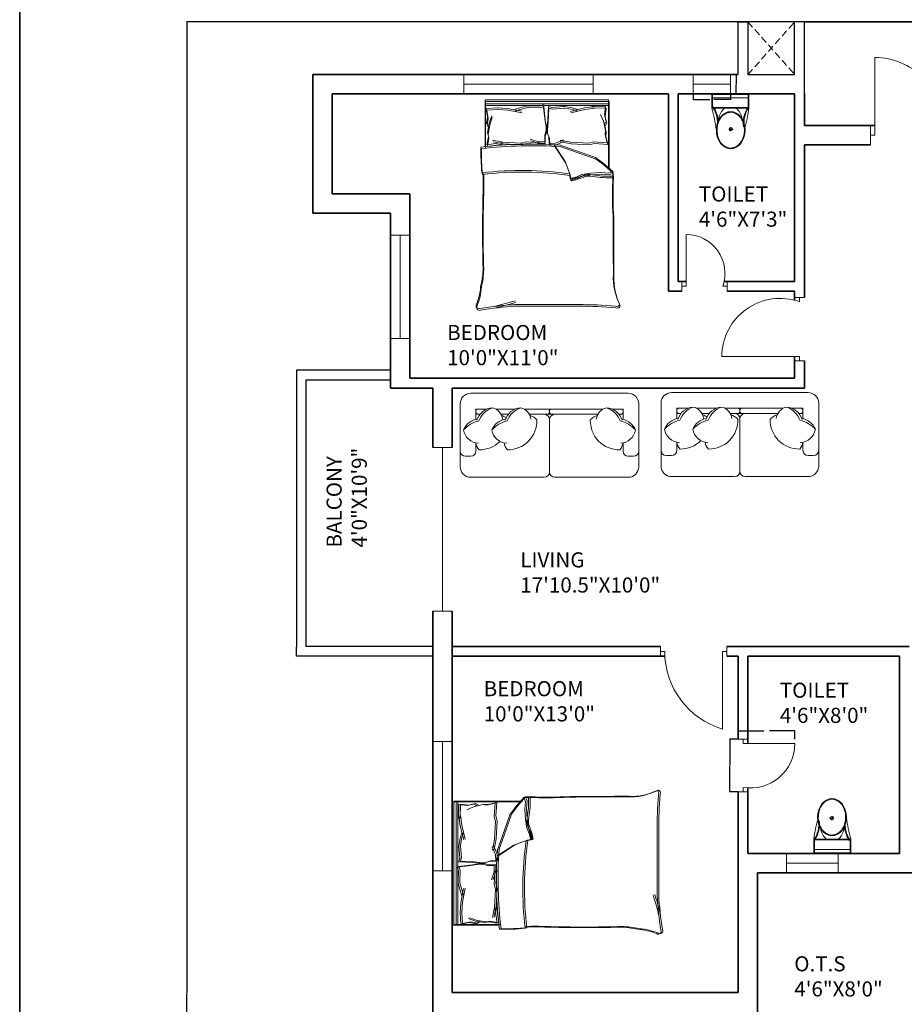
# Model space of a CAD drawing. Units: inches. Extents: x 2296 to 3812, y -1531 to 2564.
# Tile 3 of 10: x 2296 to 2706, y 1719 to 2176. Entities that reach past the tile are written whole.
import ezdxf

# ---------------------------------------------------------------- set-up
doc = ezdxf.new("R2010")
doc.units = ezdxf.units.IN
doc.linetypes.add('HIDDEN2', pattern=[4.7625, 3.175, -1.5875])
for name, color, linetype, lineweight in [('A-ANNO-DIMS', 2, 'Continuous', 18), ('A-ANNO-TTLB', 7, 'Continuous', 35), ('A-AREA-IDEN', 7, 'Continuous', 18), ('A-DOOR', 3, 'Continuous', 18), ('A-FLOR-FIXT', 9, 'Continuous', 18), ('A-FLOR-HRAL', 7, 'Continuous', 25), ('A-FURN', 8, 'Continuous', 18), ('A-GLAZ', 4, 'Continuous', 18), ('A-WALL', 7, 'Continuous', 35), ('A-WALL-HIDN', 8, 'HIDDEN2', 18)]:
    doc.layers.add(name, color=color, linetype=linetype, lineweight=lineweight)
doc.styles.get("Standard").update_dxf_attribs({"font": 'arial.ttf'})
doc.dimstyles.get("Standard").update_dxf_attribs({"dimtxt": 0.18, "dimasz": 0.18, "dimexe": 0.18, "dimexo": 0.0625, "dimgap": 0.09, "dimtad": 0, "dimtih": 1, "dimtoh": 1, "dimdec": 4, "dimzin": 0, "dimdsep": 46, "dimtxsty": 'Standard', "dimcen": 0.09, "dimadec": 0, "dimazin": 0, "dimtfac": 1, "dimtdec": 4, "dimtofl": 0, "dimtmove": 0, "dimatfit": 3, "dimfxl": 1, "dimtolj": 1, "dimtzin": 0, "dimarcsym": 0})

# ---------------------------------------------------------------- blocks, each defined once
blk = doc.blocks.new('A$C31115884')
for p, q in [((283, 498), (223, 498)), ((258, 466), (258, 523)), ((0, 200), (0, 0)), ((520, 200), (0, 200)), ((10, 190), (10, 10)), ((510, 190), (10, 190)), ((510, 10), (510, 190)), ((520, 0), (520, 200)), ((510, 54), (0, 54)), ((10, 10), (510, 10)), ((0, 0), (520, 0))]:
    blk.add_line(p, q)
blk.add_circle((256, 496), 23.6)
for centre, radius, start, end in [((2778, -205), 2807, 165.4549, 171.7133), ((-295, 403), 365, 324.2091, 9.3499), ((-295, 403), 375, 324.2091, 9.3499), ((139, 406), 293, 315.8436, 2.6563), ((806, 403), 365, 170.6501, 215.7909), ((3237, 905), 2807, 188.2867, 194.5451), ((384, 406), 293, 190.2774, 224.1564), ((806, 403), 375, 179.2036, 215.7909)]:
    blk.add_arc(centre, radius, start, end)
blk.add_ellipse((256, 510), major_axis=(0, -261), ratio=0.772727)
blk.add_open_spline([(256, 259), (263, 259), (270, 260), (288, 262), (299, 265), (320, 273), (330, 278), (350, 291), (360, 299), (378, 316), (386, 326), (402, 347), (409, 358), (421, 383), (427, 395), (436, 422), (440, 436), (445, 465), (447, 480), (448, 509), (448, 524), (445, 553), (443, 568), (436, 596), (432, 610), (422, 636), (416, 649), (402, 672), (395, 683), (379, 703), (370, 712), (351, 728), (341, 735), (321, 746), (310, 751), (289, 757), (278, 759), (256, 761), (245, 761), (223, 757), (212, 754), (191, 746), (181, 741), (161, 728), (151, 720), (133, 703), (125, 693), (110, 672), (103, 660), (90, 636), (85, 623), (76, 596), (72, 582), (67, 553), (66, 538), (64, 509), (65, 494), (68, 465), (70, 450), (77, 422), (81, 408), (91, 382), (97, 370), (111, 346), (118, 335), (135, 316), (144, 307), (162, 291), (172, 284), (193, 273), (203, 269), (225, 262), (236, 260), (250, 259), (253, 259), (256, 259)], degree=3, knots=[0, 0, 0, 0, 0.110105, 0.110105, 0.285049, 0.285049, 0.459994, 0.459994, 0.634938, 0.634938, 0.809882, 0.809882, 0.984827, 0.984827, 1.159771, 1.159771, 1.334715, 1.334715, 1.50966, 1.50966, 1.684604, 1.684604, 1.859549, 1.859549, 2.034493, 2.034493, 2.209437, 2.209437, 2.384382, 2.384382, 2.559326, 2.559326, 2.73427, 2.73427, 2.909215, 2.909215, 3.084159, 3.084159, 3.259103, 3.259103, 3.434048, 3.434048, 3.608992, 3.608992, 3.783936, 3.783936, 3.958881, 3.958881, 4.133825, 4.133825, 4.30877, 4.30877, 4.483714, 4.483714, 4.658658, 4.658658, 4.833603, 4.833603, 5.008547, 5.008547, 5.183491, 5.183491, 5.358436, 5.358436, 5.53338, 5.53338, 5.708324, 5.708324, 5.883269, 5.883269, 6.058213, 6.058213, 6.233158, 6.233158, 6.283185, 6.283185, 6.283185, 6.283185])
blk = doc.blocks.new('DOOR-BEDROOM-ENTRY-NW')
for p, q in [((33.75, 29.46), (38.25, 29.46)), ((38.25, 29.46), (36, 29.46)), ((36, 29.46), (36, 27.46)), ((36, 2), (0, 2)), ((33.75, 0), (38.25, 0)), ((36, 0), (36, 2)), ((38.25, 0), (36, 0))]:
    blk.add_line(p, q)
blk.add_arc((27, 2), 27, 70.5334, 180)
blk = doc.blocks.new('DOOR-BATH-24-NW')
for p, q in [((2, 2.25), (2, 26.25)), ((0, 4.5), (0, 0)), ((0, 0), (0, 2.25)), ((0, 2.25), (2, 2.25)), ((21.01, 2.25), (19.01, 2.25)), ((21.01, 4.5), (21.01, 0)), ((21.01, 0), (21.01, 2.25))]:
    blk.add_line(p, q)
blk.add_arc((2, 8.22), 18.03, 340.6613, 90)
blk = doc.blocks.new('DOOR-BALCONY-PAIR-N')
for p, q in [((2, 4.5), (2, 40.5)), ((64.91, 4.5), (64.91, 40.5)), ((0, 9), (0, 0)), ((66.91, 9), (66.91, 0)), ((0, 0), (0, 4.5)), ((0, 4.5), (2, 4.5)), ((66.91, 4.5), (64.91, 4.5)), ((66.91, 0), (66.91, 4.5))]:
    blk.add_line(p, q)
for centre, radius, start, end in [((2, 9.22), 31.28, 359.5901, 90), ((64.41, 9.36), 31.14, 89.0831, 180.6679)]:
    blk.add_arc(centre, radius, start, end)
blk = doc.blocks.new('DOOR-BEDROOM-36-WN')
for p, q in [((0, 38.25), (0, 33.75)), ((30.77, 38.25), (30.77, 33.75)), ((0, 33.75), (0, 36)), ((0, 36), (2, 36)), ((30.77, 36), (28.77, 36)), ((28.77, 36), (28.77, 0)), ((30.77, 33.75), (30.77, 36))]:
    blk.add_line(p, q)
blk.add_arc((39.59, 36), 37.59, 180, 253.2783)
blk = doc.blocks.new('DOOR-BATH-24-WN')
for p, q in [((0, 24.31), (4.5, 24.31)), ((4.5, 24.31), (2.25, 24.31)), ((2.25, 24.31), (2.25, 22.31)), ((2.25, 22.31), (26.25, 22.31)), ((2.25, 0), (2.25, 2)), ((4.5, 0), (0, 0)), ((0, 0), (2.25, 0))]:
    blk.add_line(p, q)
blk.add_arc((5.66, 22.31), 20.59, 260.4824, 0)
blk = doc.blocks.new('WIN-60-BEDROOM-N')
for p, q in [((0, 9), (0, 0)), ((60, 4.5), (60, 9)), ((60, 9), (60, 0)), ((0, 0), (0, 4.5)), ((0, 4.5), (60, 4.5)), ((60, 4.5), (60, 4.5))]:
    blk.add_line(p, q)
blk = doc.blocks.new('WIN-24-SHAFT-N')
for p, q in [((0, 9), (0, 0)), ((24, 4.5), (24, 9)), ((24, 9), (24, 9)), ((24, 9), (24, 0)), ((0, 0), (0, 4.5)), ((0, 4.5), (24, 4.5))]:
    blk.add_line(p, q)
blk = doc.blocks.new('WIN-60-JAMB-B')
for p, q in [((0, 60), (9, 60)), ((9, 60), (4.5, 60)), ((4.5, 60), (4.5, 0)), ((4.5, 0), (0, 0)), ((0, 0), (9, 0))]:
    blk.add_line(p, q)
blk = doc.blocks.new('WIN-17-VENT')
for p, q in [((0, 9), (0, 0)), ((17.26, 4.5), (17.26, 9)), ((17.26, 7.76), (17.26, 0)), ((0, 0), (0, 4.5)), ((0, 4.5), (0, 4.5)), ((0, 4.5), (17.26, 4.5))]:
    blk.add_line(p, q)
blk = doc.blocks.new('WIN-48-BEDROOM-NW')
for p, q in [((0, 48), (9, 48)), ((9, 48), (4.5, 48)), ((4.5, 48), (4.5, 0)), ((4.5, 0), (0, 0)), ((0, 0), (9, 0))]:
    blk.add_line(p, q)
blk = doc.blocks.new('GLAZ-BALCONY-N')
for p, q in [((0, 75.98), (9, 75.98)), ((4.5, 75.98), (4.5, 0)), ((0, 0), (9, 0))]:
    blk.add_line(p, q)
blk = doc.blocks.new('BED-DOUBLE')
for p, q in [((48.49, 95), (18.98, 95)), ((3.07, 35.36), (3.17, 33.26, 4.64)), ((5.01, 34.01), (3.17, 33.26)), ((3.17, 33.26), (7.61, 29.37)), ((8.72, 33.63), (5.01, 34.01)), ((13.37, 34.01), (8.72, 33.63)), ((17.45, 34.56), (13.37, 34.01)), ((19.86, 35.68), (17.45, 34.56)), ((22.83, 36.42), (19.86, 35.68)), ((23.21, 34.01), (22.83, 36.42)), ((25.25, 28.62), (23.21, 34.01)), ((5.09, 0), (5.09, 31.9)), ((7.61, 29.37), (11.14, 26.77)), ((30.27, 20.84), (25.25, 28.62)), ((11.14, 26.77), (17.82, 24.36)), ((17.82, 24.36), (27.82, 20.84)), ((11.92, 19.38), (5.77, 19.87)), ((5.77, 19.87), (6.7, 16.11)), ((14.27, 20.05), (11.92, 19.38)), ((22.67, 19.54), (14.27, 20.05)), ((27.51, 18.74), (22.67, 19.54)), ((29.68, 20.07), (26, 18.53)), ((32.62, 20.25), (29.68, 20.07)), ((32.82, 17.04), (32.62, 20.25)), ((34.71, 16.28), (34.71, 19.5)), ((34.71, 19.5), (37.65, 19.5)), ((43.31, 19.38), (37.16, 19.87)), ((37.65, 19.5), (41.42, 18.19)), ((45.66, 20.05), (43.31, 19.38)), ((54.06, 19.54), (45.66, 20.05)), ((54.06, 19.54), (55.42, 19.92)), ((58.9, 18.74), (54.06, 19.54)), ((55.42, 19.92), (61.53, 20.79)), ((61.53, 20.79), (60.84, 16.98)), ((62.38, 21.71), (62.38, 0)), ((6.7, 16.11), (6.47, 14.18)), ((6.47, 14.18), (7.43, 9.9)), ((33.66, 14.84), (32.82, 17.04)), ((33.75, 13.28), (33.66, 14.84)), ((34.01, 14.03), (34.71, 16.28)), ((34.01, 12.47), (34.01, 14.03)), ((61.19, 15.07), (60.49, 10.74)), ((60.84, 16.98), (61.19, 15.07)), ((6.21, 10), (6.83, 11.25)), ((6.93, 6.92), (6.21, 10)), ((7.43, 9.9), (8.85, 6.69)), ((33.01, 2.99), (33.3, 9.43)), ((33.3, 9.43), (33.75, 13.28)), ((34.71, 8.66), (34.01, 12.47)), ((60.49, 10.74), (59.28, 7.44)), ((61.71, 10.91), (61.01, 12.12)), ((61.19, 7.79), (61.71, 10.91)), ((6.47, 3.07), (6.93, 6.92)), ((16.3, 3.68), (22.8, 5.3)), ((35.4, 2.24), (34.71, 8.66)), ((52.03, 3.98), (45.45, 5.19)), ((61.88, 3.98), (61.19, 7.79)), ((62.38, 1.84), (5.09, 1.84)), ((62.38, 0), (5.09, 0)), ((6.47, 3.07), (12.95, 2.95)), ((11.75, 3.05), (16.3, 3.68)), ((12.95, 2.95), (11.75, 3.05)), ((19.55, 4.4), (22.03, 3.69)), ((22.03, 3.69), (25.54, 3.04)), ((25.54, 3.04), (25.93, 3.07)), ((25.93, 3.07), (31.24, 3.57)), ((31.24, 3.57), (33.01, 2.99)), ((37.13, 2.94), (35.4, 2.24)), ((42.46, 2.76), (37.13, 2.94)), ((42.85, 2.76), (42.46, 2.76)), ((46.31, 3.63), (42.85, 2.76)), ((48.74, 4.5), (46.31, 3.63)), ((56.62, 3.63), (52.03, 3.98)), ((56.74, 3.61), (56.62, 3.63)), ((61.87, 4), (56.74, 3.61))]:
    blk.add_line(p, q)
for centre, radius, start, end in [((40.86, 240.78), 145.97, 272.9958, 279.4091), ((65.24, 95.57), 1.31, 326.1736, 113.4781), ((1.32, 94.55), 1.32, 62.6588, 176.02), ((-24.75, 82.32), 27.65, 357.4714, 26.4681), ((17.21, 254.49), 159.5, 264.4998, 270.6351), ((87.19, -28.43), 127.63, 103.3832, 107.7053), ((92.52, 84.25), 28.25, 157.9751, 176.652), ((98.8, 77.34), 35.53, 166.0648, 178.9113), ((5471.89, 81.31), 5469.02, 180.00217, 180.28689), ((-514.68, 60.68), 578.22, 358.22771, 1.71854), ((-151.96, 43.54), 155.25, 356.9791, 3.8365), ((267.13, 37.37), 203.94, 178.4762, 181.0082), ((29.2, 1.78), 35.55, 100.6617, 109.8806), ((22.63, 36.49), 0.221, 340.2464, 91.1377), ((5.01, -7.98), 43.38, 79.8763, 92.5657), ((14.11, 42.04), 7.46, 258.6608, 293.7384), ((45.26, 187.4), 154.68, 261.7845, 276.9006), ((-35.55, 24.09), 99.87, 358.7218, 5.604), ((40.94, 218.26), 197.77, 266.0865, 276.7821)]:
    blk.add_arc(centre, radius, start, end)
blk = doc.blocks.new('*D71')
at = {"layer": 'A-ANNO-DIMS', "color": 0, "lineweight": -2, "transparency": 16777216}
for p, q in [((2629.4, 1842.2), (2629.4, 1846.25)), ((2629.58, 1846.07), (2641.22, 1846.07)), ((2655.47, 1846.07), (2643.83, 1846.07)), ((2655.65, 1842.2), (2655.65, 1846.25))]:
    blk.add_line(p, q, dxfattribs=at)
at = {"layer": 'A-ANNO-DIMS', "color": 0, "transparency": 16777216}
for points in [[(2629.58, 1846.1), (2629.58, 1846.04), (2629.4, 1846.07)], [(2655.47, 1846.1), (2655.47, 1846.04), (2655.65, 1846.07)]]:
    blk.add_solid(points, dxfattribs=at)
at = {"layer": 'Defpoints', "color": 0, "transparency": 16777216}
for p in [(2655.65, 1846.07), (2629.4, 1842.13), (2655.65, 1842.13)]:
    blk.add_point(p, dxfattribs=at)
at = {"layer": 'A-ANNO-DIMS', "color": 0, "transparency": 16777216, "insert": (2642.53, 1846.07), "char_height": 0.18, "attachment_point": 5}
blk.add_mtext('\\A1;BATH DOOR 26 TYP.', dxfattribs=at)
blk = doc.blocks.new('*D72')
at = {"layer": 'A-ANNO-DIMS', "color": 0, "lineweight": -2, "transparency": 16777216}
for p, q in [((2629.34, 1842.13), (2625.28, 1842.13)), ((2625.46, 1841.95), (2625.46, 1830.16)), ((2625.46, 1818), (2625.46, 1829.8)), ((2629.34, 1817.82), (2625.28, 1817.82))]:
    blk.add_line(p, q, dxfattribs=at)
at = {"layer": 'A-ANNO-DIMS', "color": 0, "transparency": 16777216}
for points in [[(2625.43, 1841.95), (2625.49, 1841.95), (2625.46, 1842.13)], [(2625.43, 1818), (2625.49, 1818), (2625.46, 1817.82)]]:
    blk.add_solid(points, dxfattribs=at)
at = {"layer": 'Defpoints', "color": 0, "transparency": 16777216}
for p in [(2625.46, 1842.13), (2629.4, 1842.13), (2629.4, 1817.82)]:
    blk.add_point(p, dxfattribs=at)
at = {"layer": 'A-ANNO-DIMS', "color": 0, "transparency": 16777216, "insert": (2625.46, 1829.98), "char_height": 0.18, "attachment_point": 5}
blk.add_mtext('\\A1;24 TYP.', dxfattribs=at)
blk = doc.blocks.new('*D119')
at = {"layer": 'A-ANNO-DIMS', "color": 0, "lineweight": -2, "transparency": 16777216}
for p, q in [((2608.53, 2141.6), (2608.53, 2138.89)), ((2608.71, 2139.07), (2616.25, 2139.07)), ((2625.61, 2139.07), (2618.06, 2139.07)), ((2625.79, 2141.6), (2625.79, 2138.89))]:
    blk.add_line(p, q, dxfattribs=at)
at = {"layer": 'A-ANNO-DIMS', "color": 0, "transparency": 16777216}
for points in [[(2608.71, 2139.1), (2608.71, 2139.04), (2608.53, 2139.07)], [(2625.61, 2139.1), (2625.61, 2139.04), (2625.79, 2139.07)]]:
    blk.add_solid(points, dxfattribs=at)
at = {"layer": 'Defpoints', "color": 0, "transparency": 16777216}
for p in [(2608.53, 2141.66), (2625.79, 2141.66), (2625.79, 2139.07)]:
    blk.add_point(p, dxfattribs=at)
at = {"layer": 'A-ANNO-DIMS', "color": 0, "transparency": 16777216, "insert": (2617.16, 2139.07), "char_height": 0.18, "attachment_point": 5}
blk.add_mtext('\\A1;VENT 17 TYP.', dxfattribs=at)
blk = doc.blocks.new('*D120')
at = {"layer": 'A-ANNO-DIMS', "color": 0, "lineweight": -2, "transparency": 16777216}
for p, q in [((2625.85, 2150.66), (2628.56, 2150.66)), ((2628.38, 2150.48), (2628.38, 2146.34)), ((2628.38, 2141.84), (2628.38, 2145.98)), ((2625.85, 2141.66), (2628.56, 2141.66))]:
    blk.add_line(p, q, dxfattribs=at)
at = {"layer": 'A-ANNO-DIMS', "color": 0, "transparency": 16777216}
for points in [[(2628.35, 2150.48), (2628.41, 2150.48), (2628.38, 2150.66)], [(2628.35, 2141.84), (2628.41, 2141.84), (2628.38, 2141.66)]]:
    blk.add_solid(points, dxfattribs=at)
at = {"layer": 'Defpoints', "color": 0, "transparency": 16777216}
for p in [(2625.79, 2150.66), (2628.38, 2150.66), (2625.79, 2141.66)]:
    blk.add_point(p, dxfattribs=at)
at = {"layer": 'A-ANNO-DIMS', "color": 0, "transparency": 16777216, "insert": (2628.38, 2146.16), "char_height": 0.18, "attachment_point": 5}
blk.add_mtext('\\A1;9 TYP.', dxfattribs=at)
blk = doc.blocks.new('*D128')
at = {"layer": 'A-ANNO-DIMS', "color": 0, "lineweight": -2, "transparency": 16777216}
for p, q in [((2660.01, 2175.03), (2373.54, 2175.03)), ((2373.72, 2174.85), (2373.72, 1724.41)), ((2373.72, 1273.61), (2373.72, 1724.05)), ((2666.19, 1273.43), (2373.54, 1273.43))]:
    blk.add_line(p, q, dxfattribs=at)
at = {"layer": 'A-ANNO-DIMS', "color": 0, "transparency": 16777216}
for points in [[(2373.69, 2174.85), (2373.75, 2174.85), (2373.72, 2175.03)], [(2373.69, 1273.61), (2373.75, 1273.61), (2373.72, 1273.43)]]:
    blk.add_solid(points, dxfattribs=at)
at = {"layer": 'Defpoints', "color": 0, "transparency": 16777216}
for p in [(2373.72, 2175.03), (2660.07, 2175.03), (2666.25, 1273.43)]:
    blk.add_point(p, dxfattribs=at)
at = {"layer": 'A-ANNO-DIMS', "color": 0, "transparency": 16777216, "insert": (2373.72, 1724.23), "char_height": 0.18, "attachment_point": 5}
blk.add_mtext('\\A1;901.6', dxfattribs=at)

msp = doc.modelspace()

# ---------------------------------------------------------------- linework, layer by layer
at = {"layer": 'A-ANNO-TTLB'}
msp.add_lwpolyline([(2296.1257, 2564.2989), (3812.4193, 2564.2989), (3812.4193, 1124.0028), (2296.1257, 1124.0028)], close=True, dxfattribs=at)
at = {"layer": 'A-FLOR-HRAL'}
for p, q in [((2629.4179, 2150.6578), (2629.4179, 2175.0276)), ((2629.4179, 2175.0276), (2633.9179, 2175.0276)), ((2633.9179, 2175.0276), (2633.9179, 2150.6578)), ((2655.5693, 2150.6578), (2655.5693, 2175.0276)), ((2789.0693, 2175.0276), (2655.5693, 2175.0276)), ((2660.0693, 2141.6578), (2660.0693, 2175.0276)), ((2660.0693, 2127.0276), (2660.0693, 2175.0276)), ((2660.0693, 2175.0276), (2789.0693, 2175.0276)), ((2633.9179, 2150.6578), (2655.5693, 2150.6578)), ((2633.9179, 2150.6578), (2655.5693, 2150.6578)), ((2468.0693, 2013.471), (2424.5693, 2013.471)), ((2424.5693, 2013.471), (2424.5693, 1884.8249)), ((2429.0693, 1889.3249), (2429.0693, 2008.971)), ((2429.0693, 2008.971), (2468.0693, 2008.971)), ((2429.0693, 1885.1578), (2429.0693, 1889.3249)), ((2424.5693, 1880.6578), (2424.5693, 1884.8249)), ((2487.7523, 1885.1578), (2429.0693, 1885.1578)), ((2487.7523, 1880.6578), (2424.5693, 1880.6578))]:
    msp.add_line(p, q, dxfattribs=at)
at = {"layer": 'A-FURN', "ltscale": 0.03}
for points in [[(2544.2879, 1963.7358, -0.41421356), (2541.8516, 1966.1721, -0.41421356), (2539.4153, 1963.7358), (2505.3069, 1963.7358, -0.41421356), (2500.4342, 1968.6085), (2500.4342, 1997.8443, -0.41421356), (2505.3069, 2002.7169), (2578.3963, 2002.7169, -0.41421356), (2583.269, 1997.8443), (2583.269, 1968.6085, -0.41421356), (2578.3963, 1963.7358), (2544.2879, 1963.7358, -0.41421356), (2541.8516, 1966.1721, -0.41421356), (2539.4153, 1963.7358)], [(2632.6056, 1964.0631, -0.41421356), (2630.1693, 1966.4995, -0.41421356), (2627.733, 1964.0631), (2598.4972, 1964.0631, -0.41421356), (2593.6246, 1968.9358), (2593.6246, 1998.1716, -0.41421356), (2598.4972, 2003.0442), (2661.8414, 2003.0442, -0.41421356), (2666.7141, 1998.1716), (2666.7141, 1968.9358, -0.41421356), (2661.8414, 1964.0631), (2632.6056, 1964.0631, -0.41421356), (2630.1693, 1966.4995, -0.41421356), (2627.733, 1964.0631)]]:
    msp.add_lwpolyline(points, format="xyb", dxfattribs=at)
at = {"layer": 'A-FURN'}
for points in [[(2501.9848, 1985.6857, -0.14772988), (2509.1054, 1989.8728, -0.21334276), (2515.3884, 1996.0138, -0.17866181)], [(2512.8685, 1995.4079), (2507.7432, 1995.4079), (2507.7432, 1990.62, -0.41421356)], [(2509.6024, 1992.9716), (2508.7177, 1992.9716, -0.41421356), (2507.7432, 1993.9461), (2507.7432, 1994.4334, -0.41421356), (2508.7177, 1995.4079)], [(2508.1217, 1990.2065, -0.30666349), (2515.3884, 1996.0138, -0.30632997), (2520.1355, 1990.7102, 0.87284716)], [(2508.7177, 1995.4079), (2512.8685, 1995.4079, -0.41421356)], [(2515.1091, 1985.6857, -0.14772988), (2522.2298, 1989.8728, -0.21334276), (2528.5127, 1996.0138, -0.17866181)], [(2516.9217, 1995.4079), (2525.9928, 1995.4079, -0.41421356)], [(2522.7267, 1992.9716), (2519.3749, 1992.9716, -0.41421356)], [(2521.7224, 1991.4023, 0.07186538), (2519.6798, 1992.3548, -7.11546429)], [(2520.8622, 1979.6932, 0.16554063), (2522.3694, 1976.4742, 0.42598917), (2536.0522, 1990.431, 0.12152332), (2532.8042, 1992.3548, -7.11546429)], [(2521.2461, 1990.2065, -0.30666349), (2528.5127, 1996.0138, -0.30632997), (2533.2598, 1990.7102, 0.87284716)], [(2530.046, 1995.4079), (2540.8771, 1995.4079, -0.41421356), (2541.8516, 1994.4334), (2541.8516, 1993.9461, -0.41421356), (2540.8771, 1992.9716), (2532.4992, 1992.9716, -0.41421356)], [(2539.4153, 1992.9716, -0.41421356), (2541.8516, 1990.5353)], [(2539.4153, 1992.9716, -0.41421356), (2541.8516, 1990.5353), (2541.8516, 1966.1721, -0.41421356)], [(2566.7815, 1995.4079), (2542.8261, 1995.4079, 0.41421356), (2541.8516, 1994.4334), (2541.8516, 1993.9461, 0.41421356), (2542.8261, 1992.9716), (2564.3283, 1992.9716, 0.41421356)], [(2544.2879, 1992.9716, 0.41421356), (2541.8516, 1990.5353)], [(2544.2879, 1992.9716, 0.41421356), (2541.8516, 1990.5353), (2541.8516, 1966.1721, 0.41421356)], [(2575.9653, 1979.6932, -0.16554063), (2574.4581, 1976.4742, -0.42598917), (2560.7753, 1990.431, -0.12152332), (2564.0234, 1992.3548, 7.11546429)], [(2575.5815, 1990.2065, 0.30666349), (2568.3148, 1996.0138, 0.30632997), (2563.5677, 1990.7102, -0.87284716)], [(2581.7184, 1985.6857, 0.14772988), (2574.5978, 1989.8728, 0.21334276), (2568.3148, 1996.0138, 0.17866181)], [(2574.9855, 1995.4079), (2570.8347, 1995.4079, 0.41421356)], [(2574.1008, 1992.9716), (2574.9855, 1992.9716, 0.41421356), (2575.96, 1993.9461), (2575.96, 1994.4334, 0.41421356), (2574.9855, 1995.4079)], [(2595.1751, 1986.013, -0.14772988), (2602.2958, 1990.2001, -0.21334276), (2608.5787, 1996.3411, -0.17866181)], [(2606.0589, 1995.7352), (2600.9335, 1995.7352), (2600.9335, 1990.9473, -0.41421356)], [(2602.7927, 1993.2989), (2601.908, 1993.2989, -0.41421356), (2600.9335, 1994.2735), (2600.9335, 1994.7607, -0.41421356), (2601.908, 1995.7352)], [(2601.3121, 1990.5338, -0.30666349), (2608.5787, 1996.3411, -0.30632997), (2613.3258, 1991.0375, 0.87284716)], [(2601.908, 1995.7352), (2606.0589, 1995.7352, -0.41421356)], [(2608.2995, 1986.013, -0.14772988), (2615.4201, 1990.2001, -0.21334276), (2621.7031, 1996.3411, -0.17866181)], [(2610.112, 1995.7352), (2619.1832, 1995.7352, -0.41421356)], [(2615.9171, 1993.2989), (2612.5652, 1993.2989, -0.41421356)], [(2614.9128, 1991.7296, 0.07186538), (2612.8702, 1992.6821, -7.11546429)], [(2614.0526, 1980.0206, 0.16554063), (2615.5597, 1976.8015, 0.42598917), (2629.2426, 1990.7584, 0.12152332), (2625.9945, 1992.6821, -7.11546429)], [(2614.4364, 1990.5338, -0.30666349), (2621.7031, 1996.3411, -0.30632997), (2626.4502, 1991.0375, 0.87284716)], [(2623.2363, 1995.7352), (2629.1948, 1995.7352, -0.41421356), (2630.1693, 1994.7607), (2630.1693, 1994.2735, -0.41421356), (2629.1948, 1993.2989), (2625.6896, 1993.2989, -0.41421356)], [(2627.733, 1993.2989, -0.41421356), (2630.1693, 1990.8626)], [(2627.733, 1993.2989, -0.41421356), (2630.1693, 1990.8626), (2630.1693, 1966.4995, -0.41421356)], [(2650.2266, 1995.7352), (2631.1438, 1995.7352, 0.41421356), (2630.1693, 1994.7607), (2630.1693, 1994.2735, 0.41421356), (2631.1438, 1993.2989), (2647.7734, 1993.2989, 0.41421356)], [(2632.6056, 1993.2989, 0.41421356), (2630.1693, 1990.8626)], [(2632.6056, 1993.2989, 0.41421356), (2630.1693, 1990.8626), (2630.1693, 1966.4995, 0.41421356)], [(2659.4104, 1980.0206, -0.16554063), (2657.9032, 1976.8015, -0.42598917), (2644.2204, 1990.7584, -0.12152332), (2647.4684, 1992.6821, 7.11546429)], [(2659.0266, 1990.5338, 0.30666349), (2651.7599, 1996.3411, 0.30632997), (2647.0128, 1991.0375, -0.87284716)], [(2665.1635, 1986.013, 0.14772988), (2658.0428, 1990.2001, 0.21334276), (2651.7599, 1996.3411, 0.17866181)], [(2658.4306, 1995.7352), (2654.2798, 1995.7352, 0.41421356)], [(2657.5459, 1993.2989), (2658.4306, 1993.2989, 0.41421356), (2659.4051, 1994.2735), (2659.4051, 1994.7607, 0.41421356), (2658.4306, 1995.7352)], [(2508.9658, 1979.5447, -0.35677236), (2501.9848, 1985.6857, -0.24954205), (2508.3102, 1990.7464, 9.61688035)], [(2522.0902, 1979.5447, -0.35677236), (2515.1091, 1985.6857, -0.24954205), (2521.4346, 1990.7464, 9.61688035)], [(2574.7374, 1979.5447, 0.35677236), (2581.7184, 1985.6857, 0.24954205), (2575.393, 1990.7464, -9.61688035)], [(2602.1562, 1979.872, -0.35677236), (2595.1751, 1986.013, -0.24954205), (2601.5006, 1991.0737, 9.61688035)], [(2615.2805, 1979.872, -0.35677236), (2608.2995, 1986.013, -0.24954205), (2614.6249, 1991.0737, 9.61688035)], [(2658.1825, 1979.872, 0.35677236), (2665.1635, 1986.013, 0.24954205), (2658.838, 1991.0737, -9.61688035)], [(2507.7432, 1979.6921), (2507.7432, 1975.9174, -0.41421356), (2505.3069, 1973.4811), (2502.8705, 1973.4811, -0.41421356), (2500.4342, 1975.9174)], [(2507.7379, 1979.6932, 0.16554063), (2509.2451, 1976.4742, 0.20023115), (2518.9163, 1980.3947, 0.12152332)], [(2583.269, 1975.9174, -0.41421356), (2580.8327, 1973.4811), (2578.3963, 1973.4811, -0.41421356), (2575.96, 1975.9174), (2575.96, 1979.6921)], [(2600.9335, 1980.0195), (2600.9335, 1976.2447, -0.41421356), (2598.4972, 1973.8084), (2596.0609, 1973.8084, -0.41421356), (2593.6246, 1976.2447)], [(2600.9282, 1980.0206, 0.16554063), (2602.4354, 1976.8015, 0.20023115), (2612.1067, 1980.722, 0.12152332)], [(2666.7141, 1976.2447, -0.41421356), (2664.2777, 1973.8084), (2661.8414, 1973.8084, -0.41421356), (2659.4051, 1976.2447), (2659.4051, 1980.0195)]]:
    msp.add_lwpolyline(points, format="xyb", dxfattribs=at)
for points in [[(2525.9928, 1995.4079), (2516.9217, 1995.4079)], [(2566.7815, 1995.4079), (2530.046, 1995.4079)], [(2575.96, 1990.62), (2575.96, 1995.4079), (2570.8347, 1995.4079)], [(2619.1832, 1995.7352), (2610.112, 1995.7352)], [(2650.2266, 1995.7352), (2623.2363, 1995.7352)], [(2659.4051, 1990.9473), (2659.4051, 1995.7352), (2654.2798, 1995.7352)]]:
    msp.add_lwpolyline(points, dxfattribs=at)
for points in [[(2542.8261, 1995.4079), (2540.8771, 1995.4079, -0.41421356), (2541.8516, 1994.4334), (2541.8516, 1993.9461, -0.41421356), (2540.8771, 1992.9716), (2542.8261, 1992.9716, -0.41421356), (2541.8516, 1993.9461), (2541.8516, 1994.4334, -0.41421356)], [(2631.1438, 1995.7352), (2629.1948, 1995.7352, -0.41421356), (2630.1693, 1994.7607), (2630.1693, 1994.2735, -0.41421356), (2629.1948, 1993.2989), (2631.1438, 1993.2989, -0.41421356), (2630.1693, 1994.2735), (2630.1693, 1994.7607, -0.41421356)]]:
    msp.add_lwpolyline(points, format="xyb", close=True, dxfattribs=at)
at = {"layer": 'A-WALL'}
for p, q in [((2468.0693, 2150.6578), (2432.0693, 2150.6578)), ((2432.0693, 2150.6578), (2432.0693, 2086.2649)), ((2468.0693, 2150.6578), (2629.4179, 2150.6578)), ((2468.0693, 2150.6578), (2629.4179, 2150.6578)), ((2477.0693, 2141.6578), (2441.0693, 2141.6578)), ((2441.0693, 2141.6578), (2441.0693, 2095.2649)), ((2477.0693, 2141.6578), (2597.0693, 2141.6578)), ((2597.0693, 2141.6578), (2597.0693, 2050.1578)), ((2601.5693, 2141.6578), (2601.5693, 2054.6578)), ((2601.5693, 2141.6578), (2655.5693, 2141.6578)), ((2655.5693, 2141.6578), (2655.5693, 2054.6578)), ((2660.0693, 2141.6578), (2660.0693, 2127.0276)), ((2660.0693, 2127.0276), (2692.7706, 2127.0276)), ((2660.0693, 2118.0276), (2660.0693, 2047.2032)), ((2690.7706, 2118.0276), (2660.0693, 2118.0276)), ((2441.0693, 2095.2649), (2477.0693, 2095.2649)), ((2477.0693, 2095.2649), (2477.0693, 2009.6578)), ((2432.0693, 2086.2649), (2468.0693, 2086.2649)), ((2468.0693, 2086.2649), (2468.0693, 2005.1578)), ((2468.0693, 2086.2649), (2468.0693, 2005.1578)), ((2601.5693, 2054.6578), (2605.2247, 2054.6578)), ((2622.8662, 2054.6578), (2655.5693, 2054.6578)), ((2597.0693, 2050.1578), (2603.2247, 2050.1578)), ((2624.237, 2050.1578), (2655.5693, 2050.1578)), ((2655.5693, 2050.1578), (2655.5693, 2045.8898)), ((2655.5693, 2019.7452), (2655.5693, 2009.6578)), ((2660.0693, 2017.7452), (2660.0693, 2005.1578)), ((2477.0693, 2009.6578), (2655.5693, 2009.6578)), ((2468.0693, 2005.1578), (2487.7523, 2005.1578)), ((2487.7523, 2005.1578), (2487.7523, 1977.6187)), ((2496.7523, 2005.1578), (2496.7523, 1977.6187)), ((2496.7523, 2005.1578), (2601.5693, 2005.1578)), ((2601.5693, 2005.1578), (2660.0693, 2005.1578)), ((2487.7523, 1901.6355), (2487.7523, 1540.9318)), ((2496.7523, 1901.6355), (2496.7523, 1724.6578)), ((2496.7523, 1885.1578), (2593.2843, 1885.1578)), ((2633.9, 1885.1578), (2624.0585, 1885.1578)), ((2624.0585, 1885.1578), (2708.6754, 1885.1578)), ((2496.7523, 1880.6578), (2595.3517, 1880.6578)), ((2496.7523, 1880.6578), (2595.3517, 1880.6578)), ((2624.0585, 1880.6578), (2629.4, 1880.6578)), ((2624.0585, 1880.6578), (2629.4, 1880.6578)), ((2629.4, 1880.6578), (2629.4, 1842.135)), ((2633.9, 1840.135), (2633.9, 1880.6578)), ((2633.9, 1880.6578), (2704.1754, 1880.6578)), ((2704.1754, 1847.6578), (2704.1754, 1880.6578)), ((2704.1754, 1789.1578), (2704.1754, 1847.6578)), ((2633.9, 1789.1578), (2633.9, 1819.5727)), ((2629.4, 1817.8238), (2629.4, 1724.6578)), ((2629.4, 1788.9038), (2629.4, 1788.9038)), ((2704.1754, 1789.1578), (2633.9, 1789.1578)), ((2638.4, 1780.1578), (2638.4, 1715.6578)), ((2638.4, 1780.1578), (2713.1754, 1780.1578)), ((2496.7523, 1724.6578), (2614.217, 1724.6578)), ((2629.4, 1724.6578), (2614.217, 1724.6578))]:
    msp.add_line(p, q, dxfattribs=at)
at = {"layer": 'A-WALL-HIDN'}
for p, q in [((2633.9179, 2175.0276), (2655.5693, 2150.6578)), ((2633.9179, 2150.6578), (2655.5693, 2175.0276))]:
    msp.add_line(p, q, dxfattribs=at)

# ---------------------------------------------------------------- block references
at = {"layer": 'A-DOOR'}
for name, p in [('DOOR-BALCONY-PAIR-N', (2690.771, 2118.028)), ('DOOR-BATH-24-NW', (2603.225, 2050.158)), ('DOOR-BEDROOM-ENTRY-NW', (2621.819, 2017.745)), ('DOOR-BEDROOM-36-WN', (2593.284, 1846.908)), ('DOOR-BATH-24-WN', (2629.4, 1817.824))]:
    msp.add_blockref(name, p, dxfattribs=at)
at = {"layer": 'A-FLOR-FIXT', "xscale": 0.0330640103915726, "yscale": 0.0330640103915726, "zscale": 0.0330640103915726, "rotation": 180}
msp.add_blockref('A$C31115884', (2634.3836, 2141.6578), dxfattribs=at)
at = {"layer": 'A-FLOR-FIXT', "xscale": 0.0330640103915726, "yscale": 0.0330640103915726, "zscale": 0.0330640103915726}
msp.add_blockref('A$C31115884', (2664.4093, 1789.1578), dxfattribs=at)
at = {"layer": 'A-FURN'}
for p, rotation in [((2574.3415, 2138.8402), 180), ((2574.6153, 2138.0737), 180), ((2497.5186, 1818.5551), 270), ((2496.7521, 1818.2813), 270)]:
    msp.add_blockref('BED-DOUBLE', p, dxfattribs=dict(at, rotation=rotation))
at = {"layer": 'A-GLAZ'}
for name, p in [('WIN-60-BEDROOM-N', (2502.167, 2141.658)), ('WIN-17-VENT', (2608.527, 2141.658)), ('WIN-48-BEDROOM-NW', (2468.069, 2028.125)), ('GLAZ-BALCONY-N', (2487.752, 1901.636)), ('WIN-60-JAMB-B', (2487.752, 1781.045)), ('WIN-24-SHAFT-N', (2651.784, 1780.158))]:
    msp.add_blockref(name, p, dxfattribs=at)

# ---------------------------------------------------------------- texts
at = {"layer": 'A-AREA-IDEN', "char_height": 7, "attachment_point": 1}
for s, width, insert in [('TOILET\\P4\'6"X7\'3"', 163.487917, (2611.1356, 2098.6761)), ('BEDROOM\\P10\'0"X11\'0"', 106.519629, (2494.3758, 2034.4143)), ('LIVING\\P17\'10.5"X10\'0"', 113.223621, (2528.3154, 1928.9125)), ('BEDROOM\\P10\'0"X13\'0"', 100.671801, (2511.3364, 1869.1298)), ('TOILET\\P4\'6"X8\'0"', 84.07644, (2648.7037, 1868.4122)), ('O.T.S\\P4\'6"X8\'0"', 89.687423, (2655.3869, 1741.4695))]:
    msp.add_mtext_dynamic_manual_height_columns(s, width=width, gutter_width=12.5, heights=[0], dxfattribs=dict(at, insert=insert))
at = {"layer": 'A-AREA-IDEN', "insert": (2438.4663, 1931.1209), "char_height": 7, "attachment_point": 1, "rotation": 90}
msp.add_mtext_dynamic_manual_height_columns('BALCONY\\P4\'0"X10\'9"', width=90.50646, gutter_width=12.5, heights=[0], dxfattribs=at)

# ---------------------------------------------------------------- dimensions: what is measured, and where the dimension line sits
at = {"layer": 'A-ANNO-DIMS'}
dim = msp.add_linear_dim(base=(2373.7193, 2175.0276), p1=(2666.2523, 1273.434), p2=(2660.0693, 2175.0276), angle=90, dimstyle='Standard', override={"dimdec": 1, "dimlfac": 1, "dimrnd": 0, "dimzin": 0, "dimdsep": 46, "dimlunit": 2}, dxfattribs=at)
dim.commit()
dim.dimension.update_dxf_attribs({"geometry": '*D128', "text_midpoint": (2373.7193, 1724.2308)})
for base, p1, p2, picture, middle in [((2628.376, 2150.6578), (2625.787, 2141.6578), (2625.787, 2150.6578), '*D120', (2628.376, 2146.1578)), ((2625.4625, 1842.135), (2629.4, 1817.8238), (2629.4, 1842.135), '*D72', (2625.4625, 1829.9794))]:
    dim = msp.add_linear_dim(base=base, p1=p1, p2=p2, angle=90, text='<> TYP.', dimstyle='Standard', override={"dimdec": 0, "dimlfac": 1, "dimrnd": 0, "dimzin": 0, "dimdsep": 46, "dimlunit": 2}, dxfattribs=at)
    dim.commit()
    dim.dimension.update_dxf_attribs({"geometry": picture, "text_midpoint": middle})
for base, p1, p2, text, picture, middle in [((2625.787, 2139.0688), (2608.5267, 2141.6578), (2625.787, 2141.6578), 'VENT <> TYP.', '*D119', (2617.1568, 2139.0688)), ((2655.65, 1846.0725), (2629.4, 1842.135), (2655.65, 1842.135), 'BATH DOOR <> TYP.', '*D71', (2642.525, 1846.0725))]:
    dim = msp.add_linear_dim(base=base, p1=p1, p2=p2, text=text, dimstyle='Standard', override={"dimdec": 0, "dimlfac": 1, "dimrnd": 0, "dimzin": 0, "dimdsep": 46, "dimlunit": 2}, dxfattribs=at)
    dim.commit()
    dim.dimension.update_dxf_attribs({"geometry": picture, "text_midpoint": middle})

doc.saveas('drawing.dxf')
